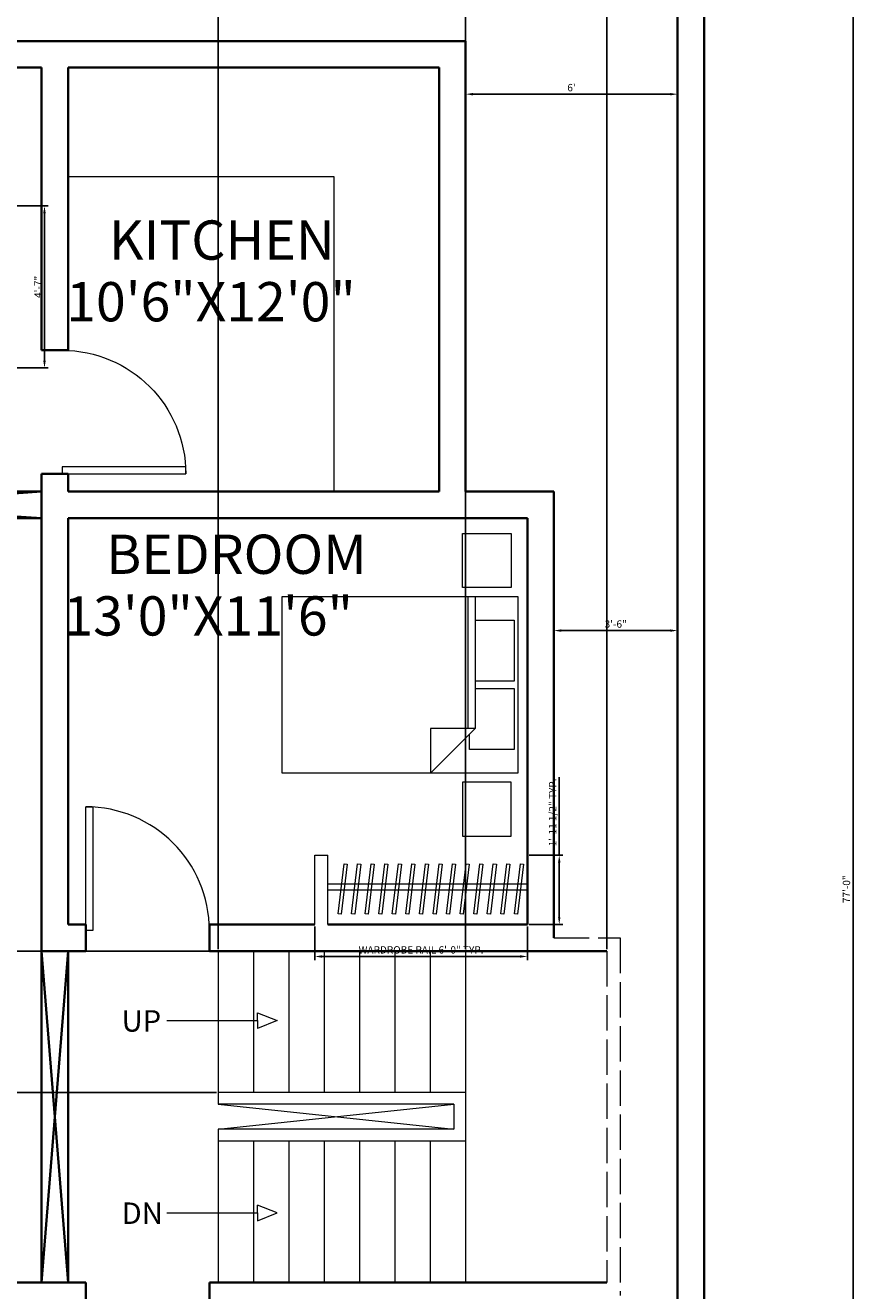
# Model space of a CAD drawing. Units: inches. Extents: x 3412 to 4225, y 13529 to 14581.
# Tile 6 of 7: x 3943 to 4225, y 13928 to 14358. Entities that reach past the tile are written whole.
import ezdxf

# ---------------------------------------------------------------- set-up
doc = ezdxf.new("R2010")
doc.units = ezdxf.units.IN
doc.linetypes.add('ACAD_ISO02W100', pattern=[15, 12, -3])
for name, color, linetype, lineweight in [('A-ANNO-DIMS', 2, 'Continuous', 13), ('A-ANNO-SYMB', 2, 'Continuous', 13), ('A-ANNO-TEXT', 7, 'Continuous', 18), ('A-AREA-IDEN', 7, 'Continuous', 18), ('A-DOOR', 4, 'Continuous', 18), ('A-FLOR-CASE', 9, 'Continuous', 18), ('A-FLOR-STRS', 3, 'Continuous', 18), ('A-FURN', 8, 'Continuous', 18), ('A-WALL', 7, 'Continuous', 35), ('A-WALL-OVHD', 8, 'ACAD_ISO02W100', 18), ('C-SITE-WALL', 7, 'Continuous', 35)]:
    doc.layers.add(name, color=color, linetype=linetype, lineweight=lineweight)
doc.styles.get("Standard").update_dxf_attribs({"font": 'arial.ttf'})
doc.dimstyles.new('ISO-25', dxfattribs={"dimtxt": 2.5, "dimasz": 2.5, "dimexe": 1.25, "dimexo": 0.625, "dimtad": 1, "dimdec": 0, "dimlunit": 3, "dimtxsty": 'Standard', "dimcen": 2.5, "dimadec": 0, "dimazin": 0, "dimtfac": 1, "dimtdec": 0, "dimtmove": 0, "dimatfit": 3, "dimfxl": 1, "dimarcsym": 0})

# ---------------------------------------------------------------- blocks, each defined once
blk = doc.blocks.new('*U3')
for p, q in [((0, 0), (0, -5)), ((30, 0), (30, -5))]:
    blk.add_line(p, q)
blk.add_lwpolyline([(0, 0), (0, 30), (1.75, 30), (1.75, 0)], close=True)
blk.add_arc((0, 0), 30, 0, 90)
blk = doc.blocks.new('Bed - Queen')
for p, q in [((0, -80.00003), (0, 0)), ((0, 0), (59.99999, 0)), ((59.99999, 0), (59.99999, -80.00003)), ((7.99999, -1.2), (28.79998, -1.2)), ((7.99999, -14.4), (7.99999, -1.2)), ((28.79998, -1.2), (28.79998, -14.4)), ((31.19999, -1.2), (51.99999, -1.2)), ((31.19999, -14.4), (31.19999, -1.2)), ((51.99999, -1.2), (51.99999, -16.4)), ((0, -14.4), (44.8, -14.4)), ((44.8, -16.8), (0, -16.8)), ((59.99999, -29.6), (44.8, -14.4)), ((44.8, -14.4), (44.8, -29.6)), ((51.99999, -16.4), (46.79936, -16.4)), ((44.8, -29.6), (59.99999, -29.6)), ((59.99999, -80.00003), (0, -80.00003))]:
    blk.add_line(p, q)
blk = doc.blocks.new('*D23')
at = {"layer": 'A-ANNO-DIMS', "color": 0, "lineweight": -2, "transparency": 16777216}
for p, q in [((4092.36, 14351.81), (4092.36, 14333.15)), ((4164.36, 14351.81), (4164.36, 14333.15)), ((4094.86, 14334.4), (4161.86, 14334.4))]:
    blk.add_line(p, q, dxfattribs=at)
at = {"layer": 'A-ANNO-DIMS', "color": 0, "transparency": 16777216}
for points in [[(4094.86, 14334.81), (4094.86, 14333.98), (4092.36, 14334.4)], [(4161.86, 14334.81), (4161.86, 14333.98), (4164.36, 14334.4)]]:
    blk.add_solid(points, dxfattribs=at)
at = {"layer": 'Defpoints', "color": 0, "transparency": 16777216}
for p in [(4092.36, 14352.43), (4164.36, 14352.43), (4164.36, 14334.4)]:
    blk.add_point(p, dxfattribs=at)
at = {"layer": 'A-ANNO-DIMS', "color": 0, "transparency": 16777216, "insert": (4128.36, 14336.3), "char_height": 2.5, "attachment_point": 5}
blk.add_mtext("6'", dxfattribs=at)
blk = doc.blocks.new('*D24')
at = {"layer": 'A-ANNO-DIMS', "color": 0, "lineweight": -2, "transparency": 16777216}
for p, q in [((4122.36, 14198.81), (4122.36, 14151)), ((4164.36, 14198.81), (4164.36, 14151)), ((4124.86, 14152.25), (4161.86, 14152.25))]:
    blk.add_line(p, q, dxfattribs=at)
at = {"layer": 'A-ANNO-DIMS', "color": 0, "transparency": 16777216}
for points in [[(4124.86, 14152.67), (4124.86, 14151.84), (4122.36, 14152.25)], [(4161.86, 14152.67), (4161.86, 14151.84), (4164.36, 14152.25)]]:
    blk.add_solid(points, dxfattribs=at)
at = {"layer": 'Defpoints', "color": 0, "transparency": 16777216}
for p in [(4122.36, 14199.43), (4164.36, 14199.43), (4164.36, 14152.25)]:
    blk.add_point(p, dxfattribs=at)
at = {"layer": 'A-ANNO-DIMS', "color": 0, "transparency": 16777216, "insert": (4143.36, 14154.16), "char_height": 2.5, "attachment_point": 5}
blk.add_mtext('3\'-6"', dxfattribs=at)
blk = doc.blocks.new('ARROW-STAIR-RUN')
for p, q in [((30.86, 2.68), (30.86, 5.34)), ((37.49, 2.68), (30.86, 5.34)), ((0, 2.68), (30.86, 2.68)), ((30.86, 2.68), (30.86, 0)), ((30.86, 0), (37.49, 2.68))]:
    blk.add_line(p, q)
blk = doc.blocks.new('NIGHTSTAND')
blk.add_lwpolyline([(0, 16.62), (18.31, 16.62), (18.31, 0), (0, 0)], close=True)
blk = doc.blocks.new('WARDROBE-RAIL-ASSEMBLY')
for p, q in [((0, 0), (0, 23.57)), ((0, 23.57), (4.5, 23.57)), ((4.5, 0), (4.5, 23.57)), ((4.5, 13.79), (72.22, 13.79)), ((4.5, 11.79), (72.22, 11.79))]:
    blk.add_line(p, q)
for points in [[(9.96, 20.59), (11, 20.47), (8.96, 3.56), (7.93, 3.68)], [(14.57, 20.59), (15.61, 20.47), (13.57, 3.56), (12.54, 3.68)], [(19.18, 20.59), (20.22, 20.47), (18.18, 3.56), (17.14, 3.68)], [(23.79, 20.59), (24.82, 20.47), (22.79, 3.56), (21.75, 3.68)], [(28.4, 20.59), (29.43, 20.47), (27.4, 3.56), (26.36, 3.68)], [(33, 20.59), (34.04, 20.47), (32, 3.56), (30.97, 3.68)], [(37.61, 20.59), (38.65, 20.47), (36.61, 3.56), (35.58, 3.68)], [(42.22, 20.59), (43.26, 20.47), (41.22, 3.56), (40.18, 3.68)], [(46.83, 20.59), (47.86, 20.47), (45.83, 3.56), (44.79, 3.68)], [(51.44, 20.59), (52.47, 20.47), (50.44, 3.56), (49.4, 3.68)], [(56.05, 20.59), (57.08, 20.47), (55.04, 3.56), (54.01, 3.68)], [(60.65, 20.59), (61.69, 20.47), (59.65, 3.56), (58.62, 3.68)], [(65.26, 20.59), (66.3, 20.47), (64.26, 3.56), (63.22, 3.68)], [(69.87, 20.59), (70.91, 20.47), (68.87, 3.56), (67.83, 3.68)]]:
    blk.add_lwpolyline(points, close=True)
blk = doc.blocks.new('*D44')
at = {"layer": 'A-ANNO-DIMS', "color": 0, "lineweight": -2, "transparency": 16777216}
for p, q in [((4041.14, 14051.81), (4041.14, 14040.35)), ((4113.36, 14051.81), (4113.36, 14040.35)), ((4043.64, 14041.6), (4110.86, 14041.6))]:
    blk.add_line(p, q, dxfattribs=at)
at = {"layer": 'A-ANNO-DIMS', "color": 0, "transparency": 16777216}
for points in [[(4043.64, 14042.02), (4043.64, 14041.18), (4041.14, 14041.6)], [(4110.86, 14042.02), (4110.86, 14041.18), (4113.36, 14041.6)]]:
    blk.add_solid(points, dxfattribs=at)
at = {"layer": 'Defpoints', "color": 0, "transparency": 16777216}
for p in [(4041.14, 14052.43), (4113.36, 14052.43), (4113.36, 14041.6)]:
    blk.add_point(p, dxfattribs=at)
at = {"layer": 'A-ANNO-DIMS', "color": 0, "transparency": 16777216, "insert": (4077.25, 14043.52), "char_height": 2.5, "attachment_point": 5}
blk.add_mtext('WARDROBE RAIL 6\'-0" TYP.', dxfattribs=at)
blk = doc.blocks.new('*D45')
at = {"layer": 'A-ANNO-DIMS', "color": 0, "lineweight": -2, "transparency": 16777216}
for p, q in [((4124.19, 14076), (4124.19, 14102.52)), ((4113.98, 14076), (4125.44, 14076)), ((4124.19, 14054.93), (4124.19, 14073.5)), ((4113.98, 14052.43), (4125.44, 14052.43))]:
    blk.add_line(p, q, dxfattribs=at)
at = {"layer": 'A-ANNO-DIMS', "color": 0, "transparency": 16777216}
for points in [[(4123.77, 14073.5), (4124.61, 14073.5), (4124.19, 14076)], [(4123.77, 14054.93), (4124.61, 14054.93), (4124.19, 14052.43)]]:
    blk.add_solid(points, dxfattribs=at)
at = {"layer": 'Defpoints', "color": 0, "transparency": 16777216}
for p in [(4113.36, 14076), (4124.19, 14076), (4113.36, 14052.43)]:
    blk.add_point(p, dxfattribs=at)
at = {"layer": 'A-ANNO-DIMS', "color": 0, "transparency": 16777216, "insert": (4122.27, 14090.51), "char_height": 2.5, "attachment_point": 5, "rotation": 90}
blk.add_mtext('1\'-11 1/2" TYP.', dxfattribs=at)
blk = doc.blocks.new('*D53')
at = {"layer": 'A-ANNO-DIMS', "color": 0, "lineweight": -2, "transparency": 16777216}
for p, q in [((3936.34, 14296.46), (3950.62, 14296.46)), ((3949.37, 14243.96), (3949.37, 14293.96)), ((3936.34, 14241.46), (3950.62, 14241.46))]:
    blk.add_line(p, q, dxfattribs=at)
at = {"layer": 'A-ANNO-DIMS', "color": 0, "transparency": 16777216}
for points in [[(3948.95, 14293.96), (3949.79, 14293.96), (3949.37, 14296.46)], [(3948.95, 14243.96), (3949.79, 14243.96), (3949.37, 14241.46)]]:
    blk.add_solid(points, dxfattribs=at)
at = {"layer": 'Defpoints', "color": 0, "transparency": 16777216}
for p in [(3935.72, 14296.46), (3949.37, 14296.46), (3935.72, 14241.46)]:
    blk.add_point(p, dxfattribs=at)
at = {"layer": 'A-ANNO-DIMS', "color": 0, "transparency": 16777216, "insert": (3947.49, 14268.96), "char_height": 2.5, "attachment_point": 5, "rotation": 90}
blk.add_mtext('4\'-7"', dxfattribs=at)
blk = doc.blocks.new('*D57')
at = {"layer": 'A-ANNO-DIMS', "color": 0, "lineweight": -2, "transparency": 16777216}
for p, q in [((4173.98, 14526.43), (4225.21, 14526.43)), ((4223.96, 13604.93), (4223.96, 14523.93)), ((4173.98, 13602.43), (4225.21, 13602.43))]:
    blk.add_line(p, q, dxfattribs=at)
at = {"layer": 'A-ANNO-DIMS', "color": 0, "transparency": 16777216}
for points in [[(4223.54, 14523.93), (4224.37, 14523.93), (4223.96, 14526.43)], [(4223.54, 13604.93), (4224.37, 13604.93), (4223.96, 13602.43)]]:
    blk.add_solid(points, dxfattribs=at)
at = {"layer": 'Defpoints', "color": 0, "transparency": 16777216}
for p in [(4173.36, 14526.43), (4223.96, 14526.43), (4173.36, 13602.43)]:
    blk.add_point(p, dxfattribs=at)
at = {"layer": 'A-ANNO-DIMS', "color": 0, "transparency": 16777216, "insert": (4222.06, 14064.43), "char_height": 2.5, "attachment_point": 5, "rotation": 90}
blk.add_mtext('77\'-0"', dxfattribs=at)
blk = doc.blocks.new('*D72')
at = {"layer": 'A-ANNO-DIMS', "color": 0, "lineweight": -2, "transparency": 16777216}
for p, q in [((3917.36, 14353.06), (3917.36, 14578.28)), ((3919.86, 14577.03), (4089.86, 14577.03)), ((4092.36, 14353.06), (4092.36, 14578.28))]:
    blk.add_line(p, q, dxfattribs=at)
at = {"layer": 'A-ANNO-DIMS', "color": 0, "transparency": 16777216}
for points in [[(3919.86, 14577.45), (3919.86, 14576.62), (3917.36, 14577.03)], [(4089.86, 14577.45), (4089.86, 14576.62), (4092.36, 14577.03)]]:
    blk.add_solid(points, dxfattribs=at)
at = {"layer": 'Defpoints', "color": 0, "transparency": 16777216}
for p in [(4092.36, 14577.03), (3917.36, 14352.43), (4092.36, 14352.43)]:
    blk.add_point(p, dxfattribs=at)
at = {"layer": 'A-ANNO-DIMS', "color": 0, "transparency": 16777216, "insert": (4004.86, 14578.91), "char_height": 2.5, "attachment_point": 5}
blk.add_mtext('14\'-7"', dxfattribs=at)
blk = doc.blocks.new('*D83')
at = {"layer": 'A-ANNO-DIMS', "color": 0, "lineweight": -2, "transparency": 16777216}
for p, q in [((4008.36, 14044.06), (4008.36, 14578.28)), ((4010.86, 14577.03), (4089.86, 14577.03)), ((4092.36, 14044.06), (4092.36, 14578.28))]:
    blk.add_line(p, q, dxfattribs=at)
at = {"layer": 'A-ANNO-DIMS', "color": 0, "transparency": 16777216}
for points in [[(4010.86, 14577.45), (4010.86, 14576.62), (4008.36, 14577.03)], [(4089.86, 14577.45), (4089.86, 14576.62), (4092.36, 14577.03)]]:
    blk.add_solid(points, dxfattribs=at)
at = {"layer": 'Defpoints', "color": 0, "transparency": 16777216}
for p in [(4092.36, 14577.03), (4008.36, 14043.43), (4092.36, 14043.43)]:
    blk.add_point(p, dxfattribs=at)
at = {"layer": 'A-ANNO-DIMS', "color": 0, "transparency": 16777216, "insert": (4050.36, 14578.93), "char_height": 2.5, "attachment_point": 5}
blk.add_mtext('7\'-0"', dxfattribs=at)
blk = doc.blocks.new('*D84')
at = {"layer": 'A-ANNO-DIMS', "color": 0, "lineweight": -2, "transparency": 16777216}
for p, q in [((4092.36, 14044.06), (4092.36, 14578.28)), ((4094.86, 14577.03), (4137.86, 14577.03)), ((4140.36, 14044.06), (4140.36, 14578.28))]:
    blk.add_line(p, q, dxfattribs=at)
at = {"layer": 'A-ANNO-DIMS', "color": 0, "transparency": 16777216}
for points in [[(4094.86, 14577.45), (4094.86, 14576.62), (4092.36, 14577.03)], [(4137.86, 14577.45), (4137.86, 14576.62), (4140.36, 14577.03)]]:
    blk.add_solid(points, dxfattribs=at)
at = {"layer": 'Defpoints', "color": 0, "transparency": 16777216}
for p in [(4140.36, 14577.03), (4092.36, 14043.43), (4140.36, 14043.43)]:
    blk.add_point(p, dxfattribs=at)
at = {"layer": 'A-ANNO-DIMS', "color": 0, "transparency": 16777216, "insert": (4116.36, 14578.93), "char_height": 2.5, "attachment_point": 5}
blk.add_mtext('4\'-0"', dxfattribs=at)
blk = doc.blocks.new('*D85')
at = {"layer": 'A-ANNO-DIMS', "color": 0, "lineweight": -2, "transparency": 16777216}
for p, q in [((4007.73, 14043.43), (3416.51, 14043.43)), ((3417.76, 13997.93), (3417.76, 14040.93)), ((4007.73, 13995.43), (3416.51, 13995.43))]:
    blk.add_line(p, q, dxfattribs=at)
at = {"layer": 'A-ANNO-DIMS', "color": 0, "transparency": 16777216}
for points in [[(3417.34, 14040.93), (3418.17, 14040.93), (3417.76, 14043.43)], [(3417.34, 13997.93), (3418.17, 13997.93), (3417.76, 13995.43)]]:
    blk.add_solid(points, dxfattribs=at)
at = {"layer": 'Defpoints', "color": 0, "transparency": 16777216}
for p in [(3417.76, 14043.43), (4008.36, 14043.43), (4008.36, 13995.43)]:
    blk.add_point(p, dxfattribs=at)
at = {"layer": 'A-ANNO-DIMS', "color": 0, "transparency": 16777216, "insert": (3415.86, 14019.43), "char_height": 2.5, "attachment_point": 5, "rotation": 90}
blk.add_mtext('4\'-0"', dxfattribs=at)

msp = doc.modelspace()

# ---------------------------------------------------------------- linework, layer by layer
at = {"layer": 'A-FLOR-CASE'}
for p, q in [((3957.36, 14306.39), (4047.67, 14306.39)), ((4047.67, 14306.39), (4047.67, 14199.43))]:
    msp.add_line(p, q, dxfattribs=at)
at = {"layer": 'A-FLOR-STRS'}
for p, q in [((4008.36, 14043.43), (4008.36, 13991.43)), ((4020.36, 14043.43), (4020.36, 13995.43)), ((4032.36, 14043.43), (4032.36, 13995.43)), ((4044.36, 14043.43), (4044.36, 13995.43)), ((4056.36, 14043.43), (4056.36, 13995.43)), ((4068.36, 14043.43), (4068.36, 13995.43)), ((4080.36, 14043.43), (4080.36, 13995.43)), ((4092.36, 14043.43), (4092.36, 13930.93)), ((4092.36, 13995.43), (4008.36, 13995.43)), ((4088.36, 13991.43), (4008.36, 13991.43)), ((4008.36, 13982.93), (4088.36, 13991.43)), ((4008.36, 13991.43), (4088.36, 13982.93)), ((4088.36, 13991.43), (4088.36, 13982.93)), ((4008.36, 13982.93), (4008.36, 13930.93)), ((4088.36, 13982.93), (4008.36, 13982.93)), ((4092.36, 13978.93), (4008.36, 13978.93)), ((4020.36, 13978.93), (4020.36, 13930.93)), ((4032.36, 13978.93), (4032.36, 13930.93)), ((4044.36, 13978.93), (4044.36, 13930.93)), ((4056.36, 13978.93), (4056.36, 13930.93)), ((4068.36, 13978.93), (4068.36, 13930.93)), ((4080.36, 13978.93), (4080.36, 13930.93))]:
    msp.add_line(p, q, dxfattribs=at)
at = {"layer": 'A-WALL'}
for p, q in [((3624.36, 14352.43), (4092.36, 14352.43)), ((4092.36, 14352.43), (4092.36, 14199.43)), ((3810.36, 14343.43), (3948.36, 14343.43)), ((3948.36, 14343.43), (3948.36, 14247.43)), ((3957.36, 14343.43), (3957.36, 14247.43)), ((3957.36, 14343.43), (4083.36, 14343.43)), ((4083.36, 14343.43), (4083.36, 14199.43)), ((3957.36, 14247.43), (3948.36, 14247.43)), ((3957.36, 14205.43), (3948.36, 14205.43)), ((3948.36, 14205.43), (3948.36, 14190.43)), ((3957.36, 14205.43), (3957.36, 14199.43)), ((3810.36, 14199.43), (3948.36, 14199.43)), ((3810.36, 14190.43), (3948.36, 14199.43)), ((3810.36, 14199.43), (3948.36, 14190.43)), ((3957.36, 14199.43), (4083.36, 14199.43)), ((4092.36, 14199.43), (4122.36, 14199.43)), ((4122.36, 14199.43), (4122.36, 14047.93)), ((3810.36, 14190.43), (3948.36, 14190.43)), ((3948.36, 14190.43), (3948.36, 14052.43)), ((3957.36, 14190.43), (4113.36, 14190.43)), ((3957.36, 14190.43), (3957.36, 14052.43)), ((4113.36, 14190.43), (4113.36, 14052.43)), ((3948.36, 14052.43), (3948.36, 13930.93)), ((3957.36, 14052.43), (3963.36, 14052.43)), ((3963.36, 14052.43), (3963.36, 14043.43)), ((4005.36, 14052.43), (4005.36, 14043.43)), ((4005.36, 14052.43), (4041.14, 14052.43)), ((4045.64, 14052.43), (4113.36, 14052.43)), ((3948.36, 14043.43), (3963.36, 14043.43)), ((3957.36, 13930.93), (3948.36, 14043.43)), ((3957.36, 14043.43), (3948.36, 13930.93)), ((3957.36, 14043.43), (3957.36, 13930.93)), ((4005.36, 14043.43), (4140.36, 14043.43)), ((3903.36, 13930.93), (3957.36, 13930.93)), ((3957.36, 13930.93), (3963.36, 13930.93)), ((3963.36, 13930.93), (3963.36, 13921.93)), ((4005.36, 13930.93), (4005.36, 13921.93)), ((4005.36, 13930.93), (4140.36, 13930.93))]:
    msp.add_line(p, q, dxfattribs=at)
at = {"layer": 'A-WALL-OVHD'}
for p, q in [((4122.36, 14047.93), (4144.86, 14047.93)), ((4144.86, 14047.93), (4144.86, 13926.43)), ((4140.36, 14043.43), (4140.36, 13930.93))]:
    msp.add_line(p, q, dxfattribs=at)
at = {"layer": 'C-SITE-WALL'}
for p, q in [((4173.36, 14526.43), (4173.36, 13602.43)), ((4164.36, 14517.43), (4164.36, 13611.43))]:
    msp.add_line(p, q, dxfattribs=at)

# ---------------------------------------------------------------- block references
at = {"layer": 'A-ANNO-SYMB', "extrusion": (0, 0, -1), "zscale": -1, "rotation": 180}
msp.add_blockref('ARROW-STAIR-RUN', (-3990.89, 14022.51), dxfattribs=at)
at = {"layer": 'A-ANNO-SYMB'}
msp.add_blockref('ARROW-STAIR-RUN', (3990.89, 13951.85), dxfattribs=at)
at = {"layer": 'A-DOOR', "xscale": -1.399999999999999, "yscale": 1.399999999999999, "zscale": 1.399999999999999}
for p, rotation in [((3955.36, 14205.43), 270), ((3963.36, 13923.93), 180)]:
    msp.add_blockref('*U3', p, dxfattribs=dict(at, rotation=rotation))
at = {"layer": 'A-DOOR', "xscale": 1.399999999999999, "yscale": 1.399999999999999, "zscale": 1.399999999999999}
msp.add_blockref('*U3', (3963.36, 14050.43), dxfattribs=at)
at = {"layer": 'A-FLOR-CASE'}
msp.add_blockref('WARDROBE-RAIL-ASSEMBLY', (4041.14, 14052.43), dxfattribs=at)
at = {"layer": 'A-FURN'}
for name, p, rotation in [('NIGHTSTAND', (4091.28, 14185.19), 270.0000000000041), ('Bed - Queen', (4110.07, 14163.83), 270)]:
    msp.add_blockref(name, p, dxfattribs=dict(at, rotation=rotation))
at = {"layer": 'A-FURN', "extrusion": (0, 0, -1), "zscale": -1, "rotation": 90.00000000000404}
msp.add_blockref('NIGHTSTAND', (-4091.28, 14082.47), dxfattribs=at)

# ---------------------------------------------------------------- texts
at = {"layer": 'A-ANNO-TEXT'}
for s, p in [('UP', (3975.55, 14016.08)), ('DN', (3975.55, 13950.78))]:
    msp.add_text(s, height=7.282, dxfattribs=at).set_placement(p)
at = {"layer": 'A-AREA-IDEN'}
for s, height, p in [('KITCHEN', 13.329, (3971.25, 14278.19)), ('10\'6"X12\'0"', 13.3293, (3956.76, 14257.26)), ('BEDROOM', 13.329, (3970.3, 14171.51)), ('13\'0"X11\'6"', 13.3293, (3955.81, 14150.57))]:
    msp.add_text(s, height=height, dxfattribs=at).set_placement(p)

# ---------------------------------------------------------------- dimensions: what is measured, and where the dimension line sits
at = {"layer": 'A-ANNO-DIMS'}
for base, p1, p2, override, picture, middle in [((4092.36, 14577.03), (3917.36, 14352.43), (4092.36, 14352.43), {"dimdec": 1, "dimlfac": 1, "dimrnd": 0, "dimzin": 1, "dimdsep": 46, "dimlunit": 4, "dimfrac": 2}, '*D72', (4004.86, 14578.91)), ((4092.36, 14577.03), (4008.36, 14043.43), (4092.36, 14043.43), {"dimdec": 1, "dimlfac": 1, "dimrnd": 0, "dimzin": 1, "dimdsep": 46, "dimlunit": 4, "dimfrac": 2}, '*D83', (4050.36, 14578.93)), ((4140.36, 14577.03), (4092.36, 14043.43), (4140.36, 14043.43), {"dimdec": 1, "dimlfac": 1, "dimrnd": 0, "dimzin": 1, "dimdsep": 46, "dimlunit": 4, "dimfrac": 2}, '*D84', (4116.36, 14578.93)), ((4164.36, 14334.4), (4092.36, 14352.43), (4164.36, 14352.43), {"dimclrd": 0, "dimclre": 0, "dimclrt": 0}, '*D23', (4128.36, 14336.3)), ((4164.36, 14152.25), (4122.36, 14199.43), (4164.36, 14199.43), {"dimclrd": 0, "dimclre": 0, "dimclrt": 0}, '*D24', (4143.36, 14154.16))]:
    dim = msp.add_linear_dim(base=base, p1=p1, p2=p2, dimstyle='ISO-25', override=override, dxfattribs=at)
    dim.commit()
    dim.dimension.update_dxf_attribs({"geometry": picture, "text_midpoint": middle})
for base, p1, p2, picture, middle in [((4223.96, 14526.43), (4173.36, 13602.43), (4173.36, 14526.43), '*D57', (4222.06, 14064.43)), ((3949.37, 14296.46), (3935.72, 14241.46), (3935.72, 14296.46), '*D53', (3947.49, 14268.96)), ((3417.76, 14043.43), (4008.36, 13995.43), (4008.36, 14043.43), '*D85', (3415.86, 14019.43))]:
    dim = msp.add_linear_dim(base=base, p1=p1, p2=p2, angle=90, dimstyle='ISO-25', override={"dimdec": 1, "dimlfac": 1, "dimrnd": 0, "dimzin": 1, "dimdsep": 46, "dimlunit": 4, "dimfrac": 2}, dxfattribs=at)
    dim.commit()
    dim.dimension.update_dxf_attribs({"geometry": picture, "text_midpoint": middle})
dim = msp.add_linear_dim(base=(4124.19, 14076), p1=(4113.36, 14052.43), p2=(4113.36, 14076), angle=90, text='<> TYP.', dimstyle='ISO-25', override={"dimdec": 1, "dimlfac": 1, "dimrnd": 0, "dimzin": 1, "dimdsep": 46, "dimlunit": 4, "dimfrac": 2}, dxfattribs=at)
dim.commit()
dim.dimension.update_dxf_attribs({"geometry": '*D45', "text_midpoint": (4122.27, 14090.51)})
dim = msp.add_linear_dim(base=(4113.36, 14041.6), p1=(4041.14, 14052.43), p2=(4113.36, 14052.43), text='WARDROBE RAIL <> TYP.', dimstyle='ISO-25', override={"dimdec": 1, "dimlfac": 1, "dimrnd": 0, "dimzin": 1, "dimdsep": 46, "dimlunit": 4, "dimfrac": 2}, dxfattribs=at)
dim.commit()
dim.dimension.update_dxf_attribs({"geometry": '*D44', "text_midpoint": (4077.25, 14043.52)})

doc.saveas('drawing.dxf')
